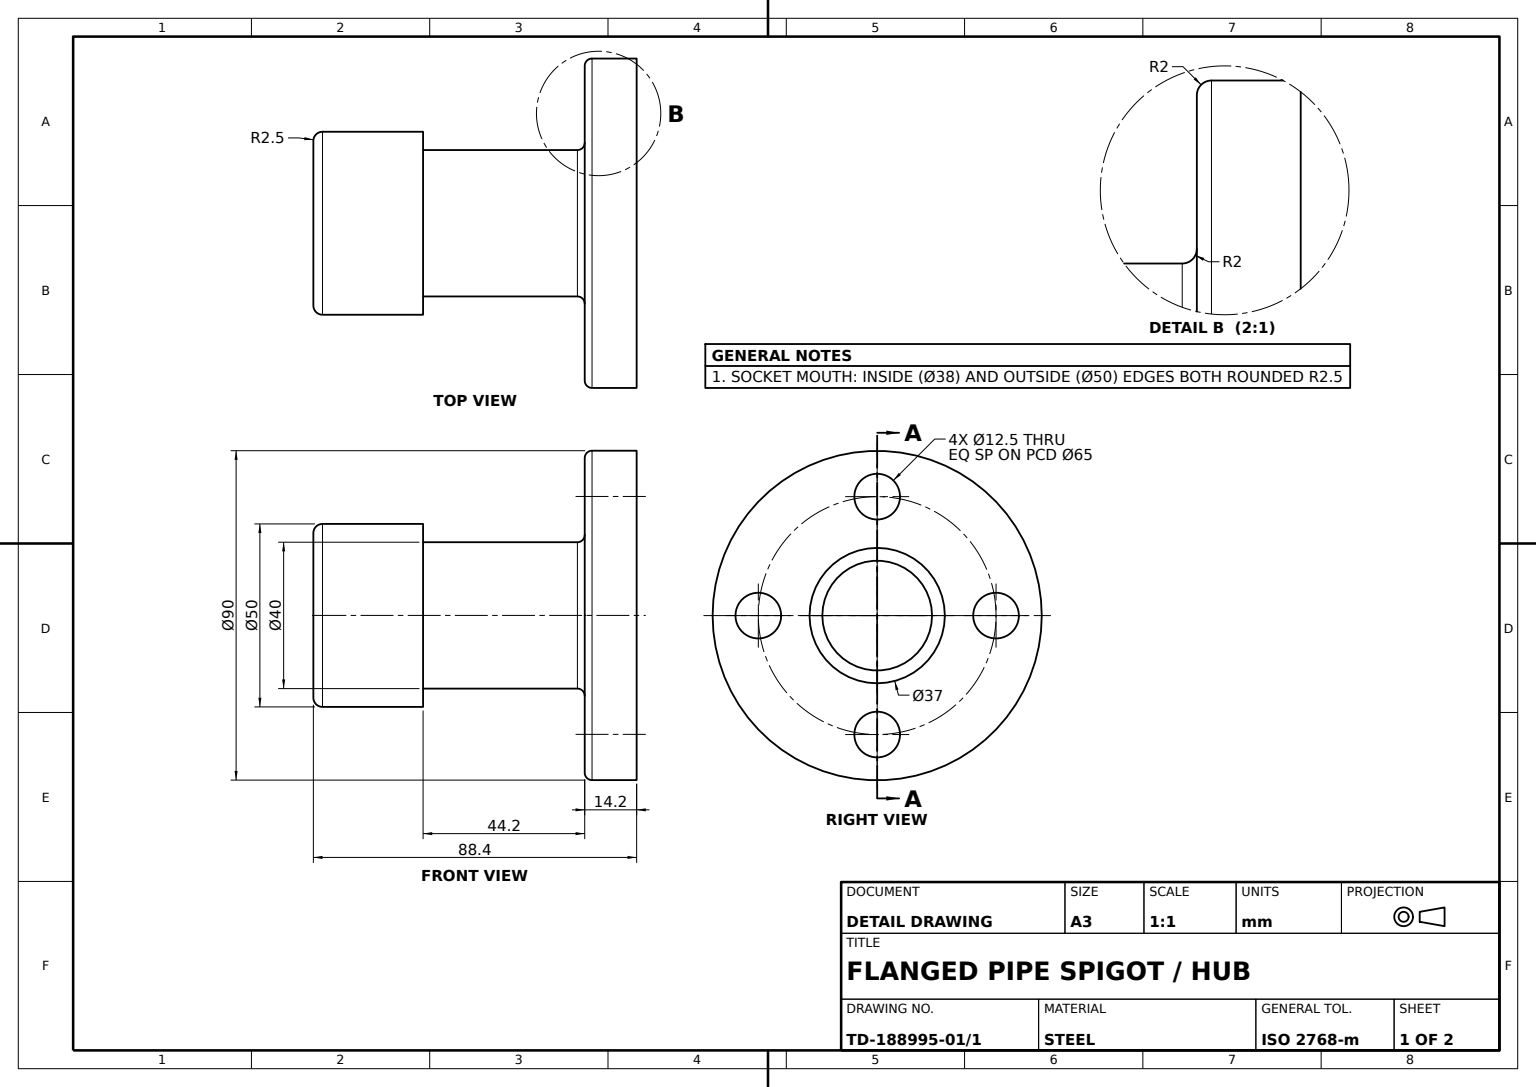
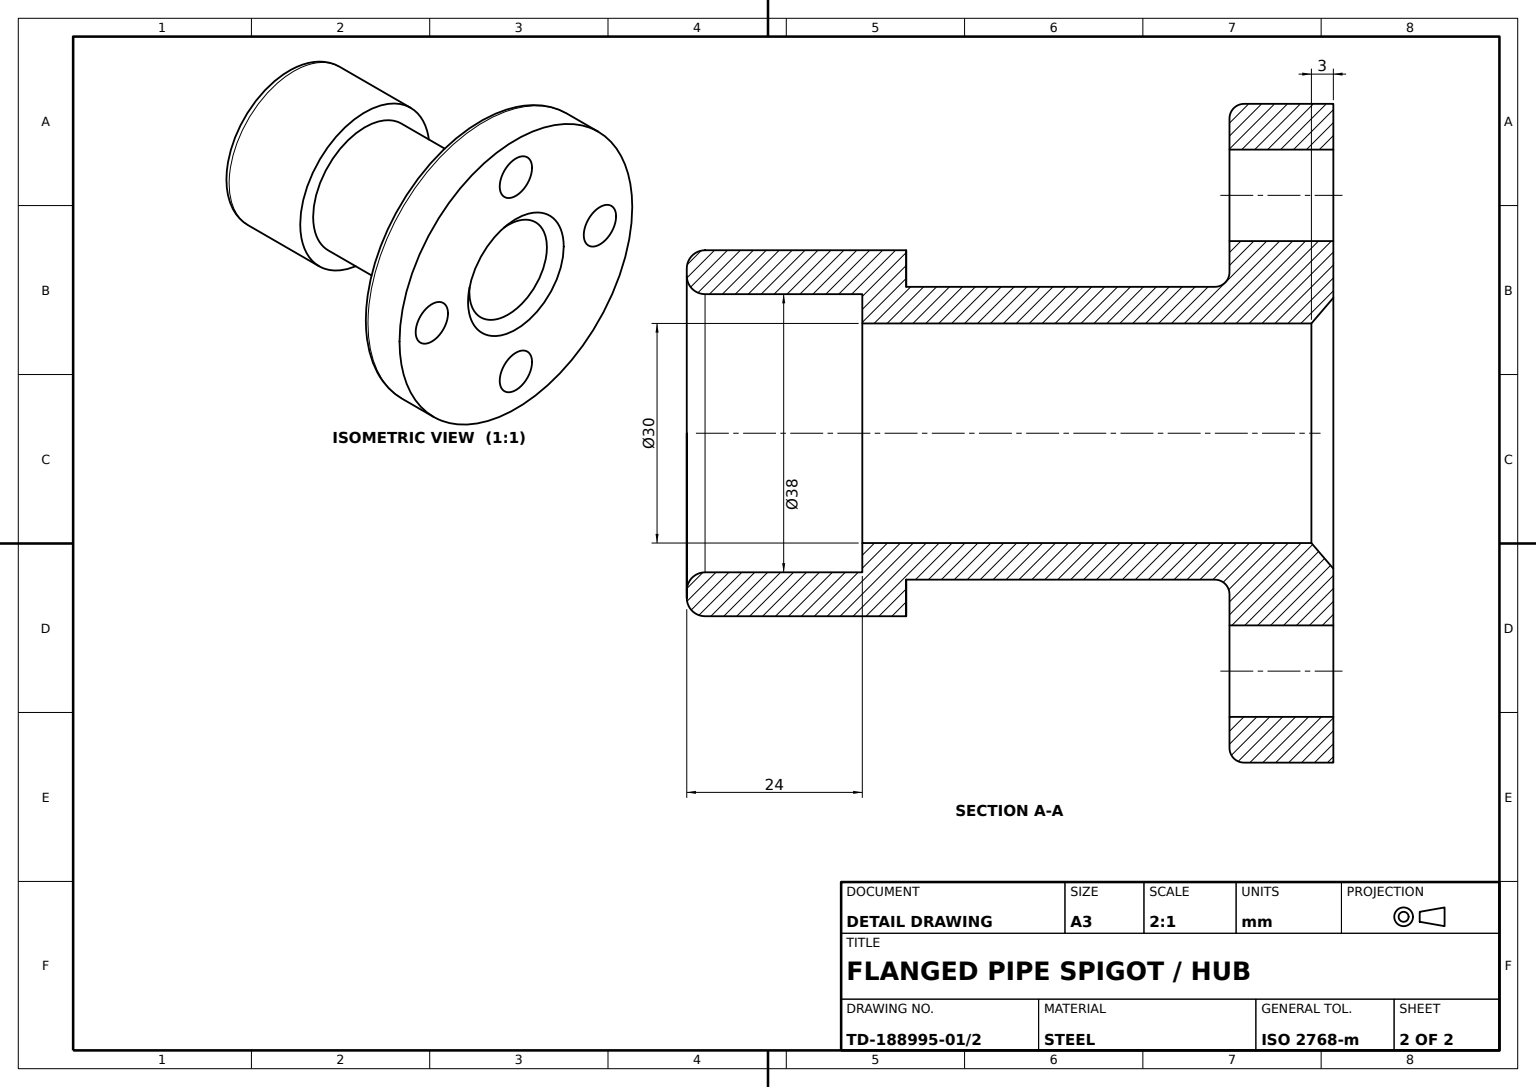
from build123d import *

# Parameters (mm, degrees)
FLANGE_PROFILE_90X_30_R     = 45
FLANGE_PROFILE_90X_30_R_2   = 15
FLANGE_90_DEPTH             = 14.2
MOUNTING_HOLES_SKETCH_R     = 6.25
FLANGE_MOUNTING_HOLES_DEPTH = 66.204601065
FLANGE_EDGE_FILLET_R2_R     = 2
HUB_PROFILE_40X_30_R        = 20
HUB_PROFILE_40X_30_R_2      = 15
HUB_40_DEPTH                = 44.2
COLLAR_PROFILE_50X_30_R     = 25
COLLAR_PROFILE_50X_30_R_2   = 15
COLLAR_50_DEPTH             = 6
SOCKET_PROFILE_50X_38_R     = 25
SOCKET_PROFILE_50X_38_R_2   = 19
SOCKET_50_DEPTH             = 24
FLANGE_CHAMFER_SIZE         = 3
FLANGE_CHAMFER_SIZE2        = 3.5
HUB_ROOT_FILLET_R2_R        = 2
SOCKET_EDGE_FILLET_R2_5_R   = 2.5


with BuildPart() as part:
    # Flange Profile Ø90xØ30 → Flange Ø90 (new body)
    with BuildSketch(Plane.XY):
        Circle(FLANGE_PROFILE_90X_30_R)
        Circle(FLANGE_PROFILE_90X_30_R_2, mode=Mode.SUBTRACT)
    extrude(amount=FLANGE_90_DEPTH)

    # Mounting Holes Sketch → Flange Mounting Holes (cut, through all)
    with BuildSketch(Plane.XY.offset(14.2)):
        with Locations((0, 32.5)):
            Circle(MOUNTING_HOLES_SKETCH_R)
        with Locations((-32.5, 0)):
            Circle(MOUNTING_HOLES_SKETCH_R)
        with Locations(Location((32.5, 0, 0), (0, 0, 180))):
            Circle(MOUNTING_HOLES_SKETCH_R)
        with Locations(Location((0, -32.5, 0), (0, 0, 180))):
            Circle(MOUNTING_HOLES_SKETCH_R)
    extrude(amount=-FLANGE_MOUNTING_HOLES_DEPTH, mode=Mode.SUBTRACT)

    # Flange Edge Fillet R2
    flange_edge_fillet_r2_edges = [part.edges().sort_by_distance(p)[0] for p in [
        (-45, 0, 14.2),
    ]]
    fillet(flange_edge_fillet_r2_edges, radius=FLANGE_EDGE_FILLET_R2_R)

    # Hub Profile Ø40xØ30 → Hub Ø40 (add)
    with BuildSketch(Plane.XY.offset(14.2)):
        Circle(HUB_PROFILE_40X_30_R)
        Circle(HUB_PROFILE_40X_30_R_2, mode=Mode.SUBTRACT)
    extrude(amount=HUB_40_DEPTH)

    # Collar Profile Ø50xØ30 → Collar Ø50 (add)
    with BuildSketch(Plane.XY.offset(58.4)):
        Circle(COLLAR_PROFILE_50X_30_R)
        Circle(COLLAR_PROFILE_50X_30_R_2, mode=Mode.SUBTRACT)
    extrude(amount=COLLAR_50_DEPTH)

    # Socket Profile Ø50xØ38 → Socket Ø50 (add)
    with BuildSketch(Plane.XY.offset(64.4)):
        Circle(SOCKET_PROFILE_50X_38_R)
        Circle(SOCKET_PROFILE_50X_38_R_2, mode=Mode.SUBTRACT)
    extrude(amount=SOCKET_50_DEPTH)

    # Flange Chamfer
    flange_chamfer_edges = [part.edges().sort_by_distance(p)[0] for p in [
        (-15, 0, 0),
    ]]
    flange_chamfer_side = [part.faces().sort_by_distance(p)[0] for p in [
        (-15, 0, 32.2),
    ]]
    chamfer(flange_chamfer_edges, length=FLANGE_CHAMFER_SIZE, length2=FLANGE_CHAMFER_SIZE2, reference=flange_chamfer_side[0])

    # Hub Root Fillet R2
    hub_root_fillet_r2_edges = [part.edges().sort_by_distance(p)[0] for p in [
        (-20, 0, 14.2),
    ]]
    fillet(hub_root_fillet_r2_edges, radius=HUB_ROOT_FILLET_R2_R)

    # Socket Edge Fillet R2.5
    socket_edge_fillet_r2_5_edges = [part.edges().sort_by_distance(p)[0] for p in [
        (-25, 0, 88.4),
        (-19, 0, 88.4),
    ]]
    fillet(socket_edge_fillet_r2_5_edges, radius=SOCKET_EDGE_FILLET_R2_5_R)


solid = part.part
